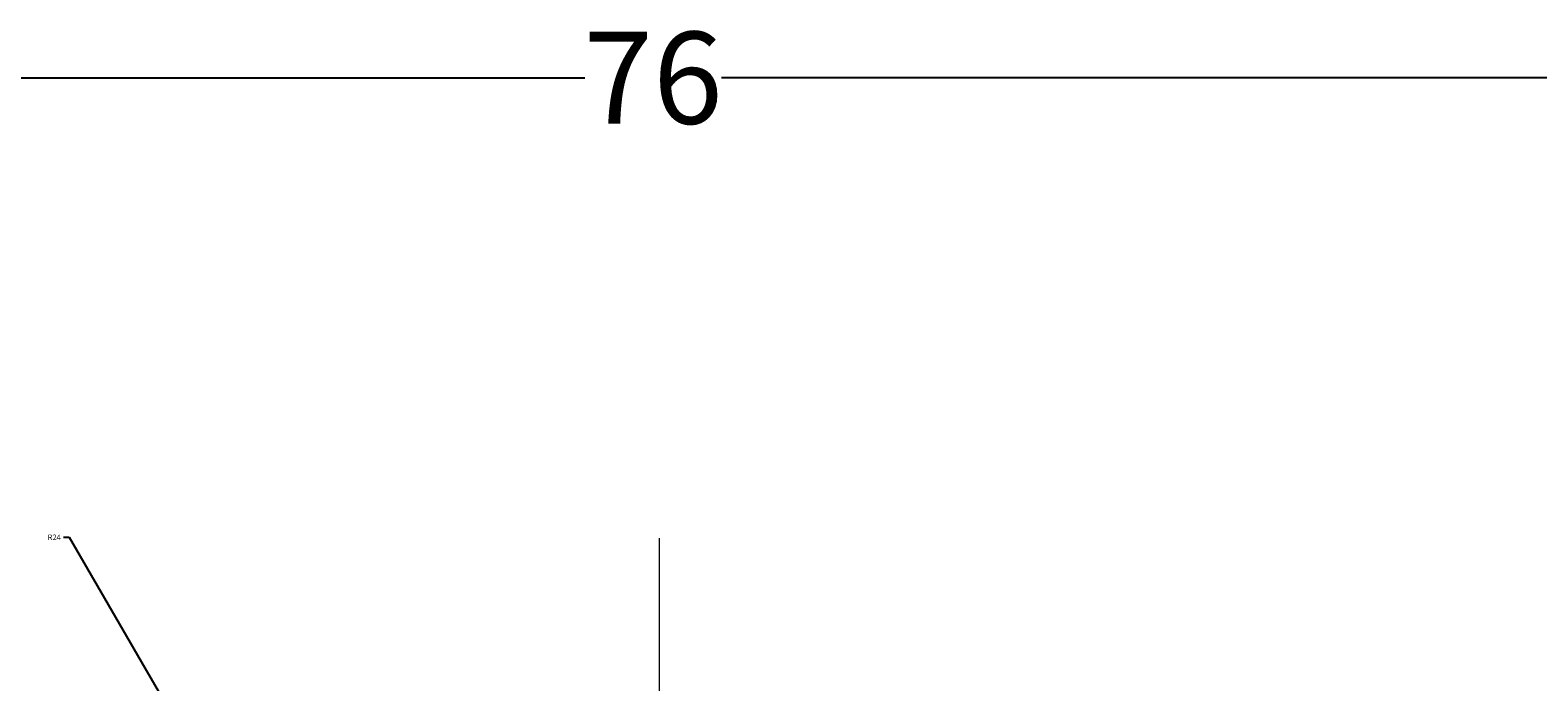
# Model space of a CAD drawing. Units: millimetres. Extents: x -50 to 109, y -46 to 152.
# Tile 17 of 18: x 13 to 62, y 131 to 152. Entities that reach past the tile are written whole.
import ezdxf

# ---------------------------------------------------------------- set-up
doc = ezdxf.new("R2010")
doc.units = ezdxf.units.MM
doc.header["$MEASUREMENT"] = 0
doc.linetypes.add('CENTER', pattern=[50.8, 31.75, -6.35, 6.35, -6.35])
doc.layers.add('M-CNTR', color=1, linetype='CENTER', lineweight=18)
doc.layers.add('M-DIMS', color=2, linetype='Continuous', lineweight=25)
doc.styles.get("Standard").update_dxf_attribs({"font": 'arial.ttf'})
doc.dimstyles.get("Standard").update_dxf_attribs({"dimtxt": 0.18, "dimasz": 0.18, "dimexe": 0.18, "dimexo": 0.0625, "dimgap": 0.09, "dimtad": 0, "dimtih": 1, "dimtoh": 1, "dimdec": 4, "dimzin": 0, "dimdsep": 46, "dimtxsty": 'Standard', "dimcen": 0.09, "dimadec": 0, "dimazin": 0, "dimtfac": 1, "dimtdec": 4, "dimtofl": 0, "dimtmove": 0, "dimatfit": 3, "dimfxl": 1, "dimtolj": 1, "dimtzin": 0, "dimarcsym": 0})

# ---------------------------------------------------------------- blocks, each defined once
blk = doc.blocks.new('*U3')
at = {"layer": 'M-CNTR', "color": 0, "transparency": 16777216}
blk.add_line((0, 2.6), (0, 33.158), dxfattribs=at)
blk = doc.blocks.new('*D7')
at = {"layer": 'Defpoints', "color": 0, "transparency": 16777216}
for p in [(70.892, 150.415), (-5.074, 114.299), (70.892, 114.299)]:
    blk.add_point(p, dxfattribs=at)
at = {"layer": 'M-DIMS', "color": 0, "lineweight": -2, "transparency": 16777216}
for p, q in [((-5.074, 114.361), (-5.074, 150.595)), ((-4.894, 150.415), (30.684, 150.415)), ((70.712, 150.415), (35.134, 150.415)), ((70.892, 114.361), (70.892, 150.595))]:
    blk.add_line(p, q, dxfattribs=at)
at = {"layer": 'M-DIMS', "color": 0, "transparency": 16777216}
for points in [[(-4.894, 150.445), (-4.894, 150.385), (-5.074, 150.415)], [(70.712, 150.445), (70.712, 150.385), (70.892, 150.415)]]:
    blk.add_solid(points, dxfattribs=at)
at = {"layer": 'M-DIMS', "color": 0, "transparency": 16777216, "insert": (32.909, 150.415), "char_height": 0.18, "attachment_point": 5}
blk.add_mtext('\\A1;{\\H16.66667x;76}', dxfattribs=at)
blk = doc.blocks.new('*D36')
at = {"layer": 'Defpoints', "color": 0, "transparency": 16777216}
for p in [(21.108, 122.986), (33.155, 102.229)]:
    blk.add_point(p, dxfattribs=at)
at = {"layer": 'M-DIMS', "color": 0, "lineweight": -2, "transparency": 16777216}
for p, q in [((13.7, 135.441), (13.88, 135.441)), ((13.88, 135.441), (21.018, 123.142)), ((33.065, 102.229), (33.245, 102.229)), ((33.155, 102.139), (33.155, 102.319))]:
    blk.add_line(p, q, dxfattribs=at)
at = {"layer": 'M-DIMS', "color": 0, "transparency": 16777216}
blk.add_solid([(21.044, 123.157), (20.992, 123.127), (21.108, 122.986)], dxfattribs=at)
at = {"layer": 'M-DIMS', "color": 0, "transparency": 16777216, "insert": (13.395, 135.441), "char_height": 0.18, "attachment_point": 5}
blk.add_mtext('\\A1;R24', dxfattribs=at)

msp = doc.modelspace()

# ---------------------------------------------------------------- block references
at = {"layer": 'M-CNTR'}
msp.add_blockref('*U3', (33.11888, 102.25066), dxfattribs=at)

# ---------------------------------------------------------------- dimensions: what is measured, and where the dimension line sits
at = {"layer": 'M-DIMS'}
dim = msp.add_linear_dim(base=(70.89158, 150.41471), p1=(-5.07376, 114.29893), p2=(70.89158, 114.29893), text='{\\H16.66667x;76}', dimstyle='Standard', override={"dimclrd": 0, "dimclre": 0, "dimclrt": 0}, dxfattribs=at)
dim.commit()
dim.dimension.update_dxf_attribs({"geometry": '*D7', "text_midpoint": (32.90891, 150.41471)})
dim = msp.add_radius_dim(center=(33.15497, 102.22852), mpoint=(21.10812, 122.98601), dimstyle='Standard', override={"dimdec": 0, "dimlfac": 1, "dimrnd": 0, "dimzin": 0, "dimdsep": 46, "dimlunit": 2}, dxfattribs=at)
dim.commit()
dim.dimension.update_dxf_attribs({"geometry": '*D36', "text_midpoint": (13.39532, 135.4405), "dimtype": 164})

doc.saveas('drawing.dxf')
